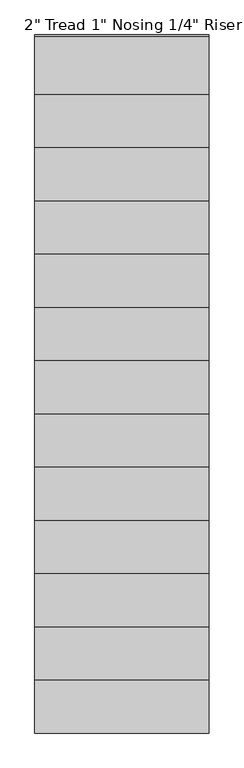
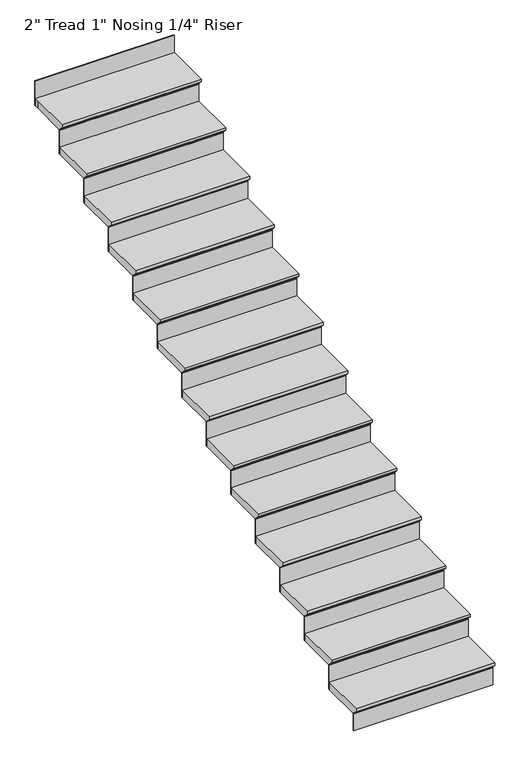
"""IFC4 building model written with IfcOpenShell, lengths in millimetres: stair flight geometry."""

from ifc_helpers import new_model, si_unit, origin, place, context, project, spatial, faceted_brep, source, transform, mapped, element, save


def stair_flight_17e69724(model_context):
    return source(origin(), model_context, "Body", "Brep", [
        faceted_brep([(-2703.0415084, -23154.3851539, 28432.9005799), (-2703.0415084, -23154.3851539, 28451.9505799), (-3617.4415084, -23154.3851539, 28451.9505799), (-3617.4415084, -23154.3851539, 28432.9005799), (-2703.0415084, -23128.9851539, 28407.5005799), (-3617.4415084, -23128.9851539, 28407.5005799), (-2703.0415084, -22849.5851539, 28451.9505799), (-3617.4415084, -22849.5851539, 28451.9505799), (-3617.4415084, -23128.9851539, 28401.1505799), (-3617.4415084, -22849.5851539, 28401.1505799), (-2703.0415084, -22849.5851539, 28401.1505799), (-2703.0415084, -23128.9851539, 28401.1505799)], [[[0, 1, 2, 3]], [[4, 0, 3, 5]], [[2, 1, 6, 7]], [[8, 9, 10, 11]], [[2, 7, 9, 8, 5, 3]], [[8, 11, 4, 5]], [[6, 1, 0, 4, 11, 10]], [[7, 6, 10, 9]]]),
        faceted_brep([(-2703.0415084, -23128.9851539, 28401.1505799), (-2703.0415084, -23128.9851539, 28282.6172466), (-2703.0415084, -23122.6351539, 28282.6172466), (-2703.0415084, -23122.6351539, 28401.1505799), (-3617.4415084, -23128.9851539, 28401.1505799), (-3617.4415084, -23122.6351539, 28401.1505799), (-3617.4415084, -23122.6351539, 28282.6172466), (-3617.4415084, -23128.9851539, 28282.6172466)], [[[0, 1, 2, 3]], [[4, 5, 6, 7]], [[1, 0, 4, 7]], [[2, 1, 7, 6]], [[3, 2, 6, 5]], [[0, 3, 5, 4]]]),
        faceted_brep([(-2703.0415084, -22849.5851539, 28570.4839133), (-2703.0415084, -22849.5851539, 28401.1505799), (-2703.0415084, -22843.2351539, 28401.1505799), (-2703.0415084, -22843.2351539, 28570.4839133), (-3617.4415084, -22849.5851539, 28570.4839133), (-3617.4415084, -22843.2351539, 28570.4839133), (-3617.4415084, -22843.2351539, 28401.1505799), (-3617.4415084, -22849.5851539, 28401.1505799)], [[[0, 1, 2, 3]], [[4, 5, 6, 7]], [[1, 0, 4, 7]], [[2, 1, 7, 6]], [[3, 2, 6, 5]], [[0, 3, 5, 4]]]),
        faceted_brep([(-3617.4415084, -22874.9851539, 28621.2839133), (-2703.0415084, -22874.9851539, 28621.2839133), (-2703.0415084, -22570.1851539, 28621.2839133), (-3617.4415084, -22570.1851539, 28621.2839133), (-3617.4415084, -22849.5851539, 28570.4839133), (-3617.4415084, -22570.1851539, 28570.4839133), (-2703.0415084, -22570.1851539, 28570.4839133), (-2703.0415084, -22849.5851539, 28570.4839133), (-3617.4415084, -22849.5851539, 28576.8339133), (-3617.4415084, -22874.9851539, 28602.2339133), (-2703.0415084, -22849.5851539, 28576.8339133), (-2703.0415084, -22874.9851539, 28602.2339133)], [[[0, 1, 2, 3]], [[4, 5, 6, 7]], [[0, 3, 5, 4, 8, 9]], [[4, 7, 10, 8]], [[2, 1, 11, 10, 7, 6]], [[3, 2, 6, 5]], [[11, 1, 0, 9]], [[10, 11, 9, 8]]]),
        faceted_brep([(-2703.0415084, -22570.1851539, 28739.8172466), (-2703.0415084, -22570.1851539, 28570.4839133), (-2703.0415084, -22563.8351539, 28570.4839133), (-2703.0415084, -22563.8351539, 28739.8172466), (-3617.4415084, -22570.1851539, 28739.8172466), (-3617.4415084, -22563.8351539, 28739.8172466), (-3617.4415084, -22563.8351539, 28570.4839133), (-3617.4415084, -22570.1851539, 28570.4839133)], [[[0, 1, 2, 3]], [[4, 5, 6, 7]], [[1, 0, 4, 7]], [[2, 1, 7, 6]], [[3, 2, 6, 5]], [[0, 3, 5, 4]]]),
        faceted_brep([(-3617.4415084, -22595.5851539, 28790.6172466), (-2703.0415084, -22595.5851539, 28790.6172466), (-2703.0415084, -22290.7851539, 28790.6172466), (-3617.4415084, -22290.7851539, 28790.6172466), (-3617.4415084, -22570.1851539, 28739.8172466), (-3617.4415084, -22290.7851539, 28739.8172466), (-2703.0415084, -22290.7851539, 28739.8172466), (-2703.0415084, -22570.1851539, 28739.8172466), (-3617.4415084, -22570.1851539, 28746.1672466), (-3617.4415084, -22595.5851539, 28771.5672466), (-2703.0415084, -22570.1851539, 28746.1672466), (-2703.0415084, -22595.5851539, 28771.5672466)], [[[0, 1, 2, 3]], [[4, 5, 6, 7]], [[0, 3, 5, 4, 8, 9]], [[4, 7, 10, 8]], [[2, 1, 11, 10, 7, 6]], [[3, 2, 6, 5]], [[11, 1, 0, 9]], [[10, 11, 9, 8]]]),
        faceted_brep([(-2703.0415084, -22290.7851539, 28909.1505799), (-2703.0415084, -22290.7851539, 28739.8172466), (-2703.0415084, -22284.4351539, 28739.8172466), (-2703.0415084, -22284.4351539, 28909.1505799), (-3617.4415084, -22290.7851539, 28909.1505799), (-3617.4415084, -22284.4351539, 28909.1505799), (-3617.4415084, -22284.4351539, 28739.8172466), (-3617.4415084, -22290.7851539, 28739.8172466)], [[[0, 1, 2, 3]], [[4, 5, 6, 7]], [[1, 0, 4, 7]], [[2, 1, 7, 6]], [[3, 2, 6, 5]], [[0, 3, 5, 4]]]),
        faceted_brep([(-3617.4415084, -22316.1851539, 28959.9505799), (-2703.0415084, -22316.1851539, 28959.9505799), (-2703.0415084, -22011.3851539, 28959.9505799), (-3617.4415084, -22011.3851539, 28959.9505799), (-3617.4415084, -22290.7851539, 28909.1505799), (-3617.4415084, -22011.3851539, 28909.1505799), (-2703.0415084, -22011.3851539, 28909.1505799), (-2703.0415084, -22290.7851539, 28909.1505799), (-3617.4415084, -22290.7851539, 28915.5005799), (-3617.4415084, -22316.1851539, 28940.9005799), (-2703.0415084, -22290.7851539, 28915.5005799), (-2703.0415084, -22316.1851539, 28940.9005799)], [[[0, 1, 2, 3]], [[4, 5, 6, 7]], [[0, 3, 5, 4, 8, 9]], [[4, 7, 10, 8]], [[2, 1, 11, 10, 7, 6]], [[3, 2, 6, 5]], [[11, 1, 0, 9]], [[10, 11, 9, 8]]]),
        faceted_brep([(-2703.0415084, -22011.3851539, 29078.4839133), (-2703.0415084, -22011.3851539, 28909.1505799), (-2703.0415084, -22005.0351539, 28909.1505799), (-2703.0415084, -22005.0351539, 29078.4839133), (-3617.4415084, -22011.3851539, 29078.4839133), (-3617.4415084, -22005.0351539, 29078.4839133), (-3617.4415084, -22005.0351539, 28909.1505799), (-3617.4415084, -22011.3851539, 28909.1505799)], [[[0, 1, 2, 3]], [[4, 5, 6, 7]], [[1, 0, 4, 7]], [[2, 1, 7, 6]], [[3, 2, 6, 5]], [[0, 3, 5, 4]]]),
        faceted_brep([(-3617.4415084, -22036.7851539, 29129.2839133), (-2703.0415084, -22036.7851539, 29129.2839133), (-2703.0415084, -21731.9851539, 29129.2839133), (-3617.4415084, -21731.9851539, 29129.2839133), (-3617.4415084, -22011.3851539, 29078.4839133), (-3617.4415084, -21731.9851539, 29078.4839133), (-2703.0415084, -21731.9851539, 29078.4839133), (-2703.0415084, -22011.3851539, 29078.4839133), (-3617.4415084, -22011.3851539, 29084.8339133), (-3617.4415084, -22036.7851539, 29110.2339133), (-2703.0415084, -22011.3851539, 29084.8339133), (-2703.0415084, -22036.7851539, 29110.2339133)], [[[0, 1, 2, 3]], [[4, 5, 6, 7]], [[0, 3, 5, 4, 8, 9]], [[4, 7, 10, 8]], [[2, 1, 11, 10, 7, 6]], [[3, 2, 6, 5]], [[11, 1, 0, 9]], [[10, 11, 9, 8]]]),
        faceted_brep([(-2703.0415084, -21731.9851539, 29247.8172466), (-2703.0415084, -21731.9851539, 29078.4839133), (-2703.0415084, -21725.6351539, 29078.4839133), (-2703.0415084, -21725.6351539, 29247.8172466), (-3617.4415084, -21731.9851539, 29247.8172466), (-3617.4415084, -21725.6351539, 29247.8172466), (-3617.4415084, -21725.6351539, 29078.4839133), (-3617.4415084, -21731.9851539, 29078.4839133)], [[[0, 1, 2, 3]], [[4, 5, 6, 7]], [[1, 0, 4, 7]], [[2, 1, 7, 6]], [[3, 2, 6, 5]], [[0, 3, 5, 4]]]),
        faceted_brep([(-3617.4415084, -21757.3851539, 29298.6172466), (-2703.0415084, -21757.3851539, 29298.6172466), (-2703.0415084, -21452.5851539, 29298.6172466), (-3617.4415084, -21452.5851539, 29298.6172466), (-3617.4415084, -21731.9851539, 29247.8172466), (-3617.4415084, -21452.5851539, 29247.8172466), (-2703.0415084, -21452.5851539, 29247.8172466), (-2703.0415084, -21731.9851539, 29247.8172466), (-3617.4415084, -21731.9851539, 29254.1672466), (-3617.4415084, -21757.3851539, 29279.5672466), (-2703.0415084, -21731.9851539, 29254.1672466), (-2703.0415084, -21757.3851539, 29279.5672466)], [[[0, 1, 2, 3]], [[4, 5, 6, 7]], [[0, 3, 5, 4, 8, 9]], [[4, 7, 10, 8]], [[2, 1, 11, 10, 7, 6]], [[3, 2, 6, 5]], [[11, 1, 0, 9]], [[10, 11, 9, 8]]]),
        faceted_brep([(-2703.0415084, -21452.5851539, 29417.1505799), (-2703.0415084, -21452.5851539, 29247.8172466), (-2703.0415084, -21446.2351539, 29247.8172466), (-2703.0415084, -21446.2351539, 29417.1505799), (-3617.4415084, -21452.5851539, 29417.1505799), (-3617.4415084, -21446.2351539, 29417.1505799), (-3617.4415084, -21446.2351539, 29247.8172466), (-3617.4415084, -21452.5851539, 29247.8172466)], [[[0, 1, 2, 3]], [[4, 5, 6, 7]], [[1, 0, 4, 7]], [[2, 1, 7, 6]], [[3, 2, 6, 5]], [[0, 3, 5, 4]]]),
        faceted_brep([(-3617.4415084, -21477.9851539, 29467.9505799), (-2703.0415084, -21477.9851539, 29467.9505799), (-2703.0415084, -21173.1851539, 29467.9505799), (-3617.4415084, -21173.1851539, 29467.9505799), (-3617.4415084, -21452.5851539, 29417.1505799), (-3617.4415084, -21173.1851539, 29417.1505799), (-2703.0415084, -21173.1851539, 29417.1505799), (-2703.0415084, -21452.5851539, 29417.1505799), (-3617.4415084, -21452.5851539, 29423.5005799), (-3617.4415084, -21477.9851539, 29448.9005799), (-2703.0415084, -21452.5851539, 29423.5005799), (-2703.0415084, -21477.9851539, 29448.9005799)], [[[0, 1, 2, 3]], [[4, 5, 6, 7]], [[0, 3, 5, 4, 8, 9]], [[4, 7, 10, 8]], [[2, 1, 11, 10, 7, 6]], [[3, 2, 6, 5]], [[11, 1, 0, 9]], [[10, 11, 9, 8]]]),
        faceted_brep([(-2703.0415084, -21173.1851539, 29586.4839133), (-2703.0415084, -21173.1851539, 29417.1505799), (-2703.0415084, -21166.8351539, 29417.1505799), (-2703.0415084, -21166.8351539, 29586.4839133), (-3617.4415084, -21173.1851539, 29586.4839133), (-3617.4415084, -21166.8351539, 29586.4839133), (-3617.4415084, -21166.8351539, 29417.1505799), (-3617.4415084, -21173.1851539, 29417.1505799)], [[[0, 1, 2, 3]], [[4, 5, 6, 7]], [[1, 0, 4, 7]], [[2, 1, 7, 6]], [[3, 2, 6, 5]], [[0, 3, 5, 4]]]),
        faceted_brep([(-3617.4415084, -21198.5851539, 29637.2839133), (-2703.0415084, -21198.5851539, 29637.2839133), (-2703.0415084, -20893.7851539, 29637.2839133), (-3617.4415084, -20893.7851539, 29637.2839133), (-3617.4415084, -21173.1851539, 29586.4839133), (-3617.4415084, -20893.7851539, 29586.4839133), (-2703.0415084, -20893.7851539, 29586.4839133), (-2703.0415084, -21173.1851539, 29586.4839133), (-3617.4415084, -21173.1851539, 29592.8339133), (-3617.4415084, -21198.5851539, 29618.2339133), (-2703.0415084, -21173.1851539, 29592.8339133), (-2703.0415084, -21198.5851539, 29618.2339133)], [[[0, 1, 2, 3]], [[4, 5, 6, 7]], [[0, 3, 5, 4, 8, 9]], [[4, 7, 10, 8]], [[2, 1, 11, 10, 7, 6]], [[3, 2, 6, 5]], [[11, 1, 0, 9]], [[10, 11, 9, 8]]]),
        faceted_brep([(-2703.0415084, -20893.7851539, 29755.8172466), (-2703.0415084, -20893.7851539, 29586.4839133), (-2703.0415084, -20887.4351539, 29586.4839133), (-2703.0415084, -20887.4351539, 29755.8172466), (-3617.4415084, -20893.7851539, 29755.8172466), (-3617.4415084, -20887.4351539, 29755.8172466), (-3617.4415084, -20887.4351539, 29586.4839133), (-3617.4415084, -20893.7851539, 29586.4839133)], [[[0, 1, 2, 3]], [[4, 5, 6, 7]], [[1, 0, 4, 7]], [[2, 1, 7, 6]], [[3, 2, 6, 5]], [[0, 3, 5, 4]]]),
        faceted_brep([(-3617.4415084, -20919.1851539, 29806.6172466), (-2703.0415084, -20919.1851539, 29806.6172466), (-2703.0415084, -20614.3851539, 29806.6172466), (-3617.4415084, -20614.3851539, 29806.6172466), (-3617.4415084, -20893.7851539, 29755.8172466), (-3617.4415084, -20614.3851539, 29755.8172466), (-2703.0415084, -20614.3851539, 29755.8172466), (-2703.0415084, -20893.7851539, 29755.8172466), (-3617.4415084, -20893.7851539, 29762.1672466), (-3617.4415084, -20919.1851539, 29787.5672466), (-2703.0415084, -20893.7851539, 29762.1672466), (-2703.0415084, -20919.1851539, 29787.5672466)], [[[0, 1, 2, 3]], [[4, 5, 6, 7]], [[0, 3, 5, 4, 8, 9]], [[4, 7, 10, 8]], [[2, 1, 11, 10, 7, 6]], [[3, 2, 6, 5]], [[11, 1, 0, 9]], [[10, 11, 9, 8]]]),
        faceted_brep([(-2703.0415084, -20614.3851539, 29925.1505799), (-2703.0415084, -20614.3851539, 29755.8172466), (-2703.0415084, -20608.0351539, 29755.8172466), (-2703.0415084, -20608.0351539, 29925.1505799), (-3617.4415084, -20614.3851539, 29925.1505799), (-3617.4415084, -20608.0351539, 29925.1505799), (-3617.4415084, -20608.0351539, 29755.8172466), (-3617.4415084, -20614.3851539, 29755.8172466)], [[[0, 1, 2, 3]], [[4, 5, 6, 7]], [[1, 0, 4, 7]], [[2, 1, 7, 6]], [[3, 2, 6, 5]], [[0, 3, 5, 4]]]),
        faceted_brep([(-3617.4415084, -20639.7851539, 29975.9505799), (-2703.0415084, -20639.7851539, 29975.9505799), (-2703.0415084, -20334.9851539, 29975.9505799), (-3617.4415084, -20334.9851539, 29975.9505799), (-3617.4415084, -20614.3851539, 29925.1505799), (-3617.4415084, -20334.9851539, 29925.1505799), (-2703.0415084, -20334.9851539, 29925.1505799), (-2703.0415084, -20614.3851539, 29925.1505799), (-3617.4415084, -20614.3851539, 29931.5005799), (-3617.4415084, -20639.7851539, 29956.9005799), (-2703.0415084, -20614.3851539, 29931.5005799), (-2703.0415084, -20639.7851539, 29956.9005799)], [[[0, 1, 2, 3]], [[4, 5, 6, 7]], [[0, 3, 5, 4, 8, 9]], [[4, 7, 10, 8]], [[2, 1, 11, 10, 7, 6]], [[3, 2, 6, 5]], [[11, 1, 0, 9]], [[10, 11, 9, 8]]]),
        faceted_brep([(-2703.0415084, -20334.9851539, 30094.4839133), (-2703.0415084, -20334.9851539, 29925.1505799), (-2703.0415084, -20328.6351539, 29925.1505799), (-2703.0415084, -20328.6351539, 30094.4839133), (-3617.4415084, -20334.9851539, 30094.4839133), (-3617.4415084, -20328.6351539, 30094.4839133), (-3617.4415084, -20328.6351539, 29925.1505799), (-3617.4415084, -20334.9851539, 29925.1505799)], [[[0, 1, 2, 3]], [[4, 5, 6, 7]], [[1, 0, 4, 7]], [[2, 1, 7, 6]], [[3, 2, 6, 5]], [[0, 3, 5, 4]]]),
        faceted_brep([(-3617.4415084, -20360.3851539, 30145.2839133), (-2703.0415084, -20360.3851539, 30145.2839133), (-2703.0415084, -20055.5851539, 30145.2839133), (-3617.4415084, -20055.5851539, 30145.2839133), (-3617.4415084, -20334.9851539, 30094.4839133), (-3617.4415084, -20055.5851539, 30094.4839133), (-2703.0415084, -20055.5851539, 30094.4839133), (-2703.0415084, -20334.9851539, 30094.4839133), (-3617.4415084, -20334.9851539, 30100.8339133), (-3617.4415084, -20360.3851539, 30126.2339133), (-2703.0415084, -20334.9851539, 30100.8339133), (-2703.0415084, -20360.3851539, 30126.2339133)], [[[0, 1, 2, 3]], [[4, 5, 6, 7]], [[0, 3, 5, 4, 8, 9]], [[4, 7, 10, 8]], [[2, 1, 11, 10, 7, 6]], [[3, 2, 6, 5]], [[11, 1, 0, 9]], [[10, 11, 9, 8]]]),
        faceted_brep([(-2703.0415084, -20055.5851539, 30263.8172466), (-2703.0415084, -20055.5851539, 30094.4839133), (-2703.0415084, -20049.2351539, 30094.4839133), (-2703.0415084, -20049.2351539, 30263.8172466), (-3617.4415084, -20055.5851539, 30263.8172466), (-3617.4415084, -20049.2351539, 30263.8172466), (-3617.4415084, -20049.2351539, 30094.4839133), (-3617.4415084, -20055.5851539, 30094.4839133)], [[[0, 1, 2, 3]], [[4, 5, 6, 7]], [[1, 0, 4, 7]], [[2, 1, 7, 6]], [[3, 2, 6, 5]], [[0, 3, 5, 4]]]),
        faceted_brep([(-3617.4415084, -20080.9851539, 30314.6172466), (-2703.0415084, -20080.9851539, 30314.6172466), (-2703.0415084, -19776.1851539, 30314.6172466), (-3617.4415084, -19776.1851539, 30314.6172466), (-3617.4415084, -20055.5851539, 30263.8172466), (-3617.4415084, -19776.1851539, 30263.8172466), (-2703.0415084, -19776.1851539, 30263.8172466), (-2703.0415084, -20055.5851539, 30263.8172466), (-3617.4415084, -20055.5851539, 30270.1672466), (-3617.4415084, -20080.9851539, 30295.5672466), (-2703.0415084, -20055.5851539, 30270.1672466), (-2703.0415084, -20080.9851539, 30295.5672466)], [[[0, 1, 2, 3]], [[4, 5, 6, 7]], [[0, 3, 5, 4, 8, 9]], [[4, 7, 10, 8]], [[2, 1, 11, 10, 7, 6]], [[3, 2, 6, 5]], [[11, 1, 0, 9]], [[10, 11, 9, 8]]]),
        faceted_brep([(-2703.0415084, -19496.7851539, 30602.4839133), (-2703.0415084, -19496.7851539, 30433.1505799), (-2703.0415084, -19490.4351539, 30433.1505799), (-2703.0415084, -19490.4351539, 30602.4839133), (-3617.4415084, -19496.7851539, 30602.4839133), (-3617.4415084, -19490.4351539, 30602.4839133), (-3617.4415084, -19490.4351539, 30433.1505799), (-3617.4415084, -19496.7851539, 30433.1505799)], [[[0, 1, 2, 3]], [[4, 5, 6, 7]], [[1, 0, 4, 7]], [[2, 1, 7, 6]], [[3, 2, 6, 5]], [[0, 3, 5, 4]]]),
        faceted_brep([(-2703.0415084, -19776.1851539, 30433.1505799), (-2703.0415084, -19776.1851539, 30263.8172466), (-2703.0415084, -19769.8351539, 30263.8172466), (-2703.0415084, -19769.8351539, 30433.1505799), (-3617.4415084, -19776.1851539, 30433.1505799), (-3617.4415084, -19769.8351539, 30433.1505799), (-3617.4415084, -19769.8351539, 30263.8172466), (-3617.4415084, -19776.1851539, 30263.8172466)], [[[0, 1, 2, 3]], [[4, 5, 6, 7]], [[1, 0, 4, 7]], [[2, 1, 7, 6]], [[3, 2, 6, 5]], [[0, 3, 5, 4]]]),
        faceted_brep([(-3617.4415084, -19496.7851539, 30483.9505799), (-3617.4415084, -19522.1851539, 30483.9505799), (-3617.4415084, -19801.5851539, 30483.9505799), (-2703.0415084, -19801.5851539, 30483.9505799), (-2703.0415084, -19496.7851539, 30483.9505799), (-3617.4415084, -19522.1851539, 30433.1505799), (-3617.4415084, -19496.7851539, 30433.1505799), (-2703.0415084, -19496.7851539, 30433.1505799), (-2703.0415084, -19776.1851539, 30433.1505799), (-3617.4415084, -19776.1851539, 30433.1505799), (-3617.4415084, -19776.1851539, 30439.5005799), (-3617.4415084, -19801.5851539, 30464.9005799), (-2703.0415084, -19776.1851539, 30439.5005799), (-2703.0415084, -19801.5851539, 30464.9005799)], [[[0, 1, 2, 3, 4]], [[5, 6, 7, 8, 9]], [[1, 0, 6, 5]], [[2, 1, 5, 9, 10, 11]], [[9, 8, 12, 10]], [[4, 3, 13, 12, 8, 7]], [[0, 4, 7, 6]], [[13, 3, 2, 11]], [[12, 13, 11, 10]]]),
    ])


if __name__ == "__main__":
    model = new_model("IFC4")
    model_context = context("Model", 3, world=origin())
    ifc_project = project(units=[si_unit("LENGTHUNIT", "METRE", prefix="MILLI")], contexts=[model_context])
    site = spatial("IfcSite", under=ifc_project)
    building = spatial("IfcBuilding", under=site)
    placement = place(None, origin())
    stair_flight_shape = stair_flight_17e69724(model_context)
    element("IfcStairFlight", 1, ObjectType="2\" Tread 1\" Nosing 1/4\" Riser", at=placement, inside=building, context=model_context, shape_type="MappedRepresentation", body=[
        mapped(stair_flight_shape, transform((0.0, 0.0, 0.0), x_axis=(1.0, 0.0, 0.0), y_axis=(0.0, 1.0, 0.0), z_axis=(0.0, 0.0, 1.0))),
    ])
    save(model, "model.ifc")
